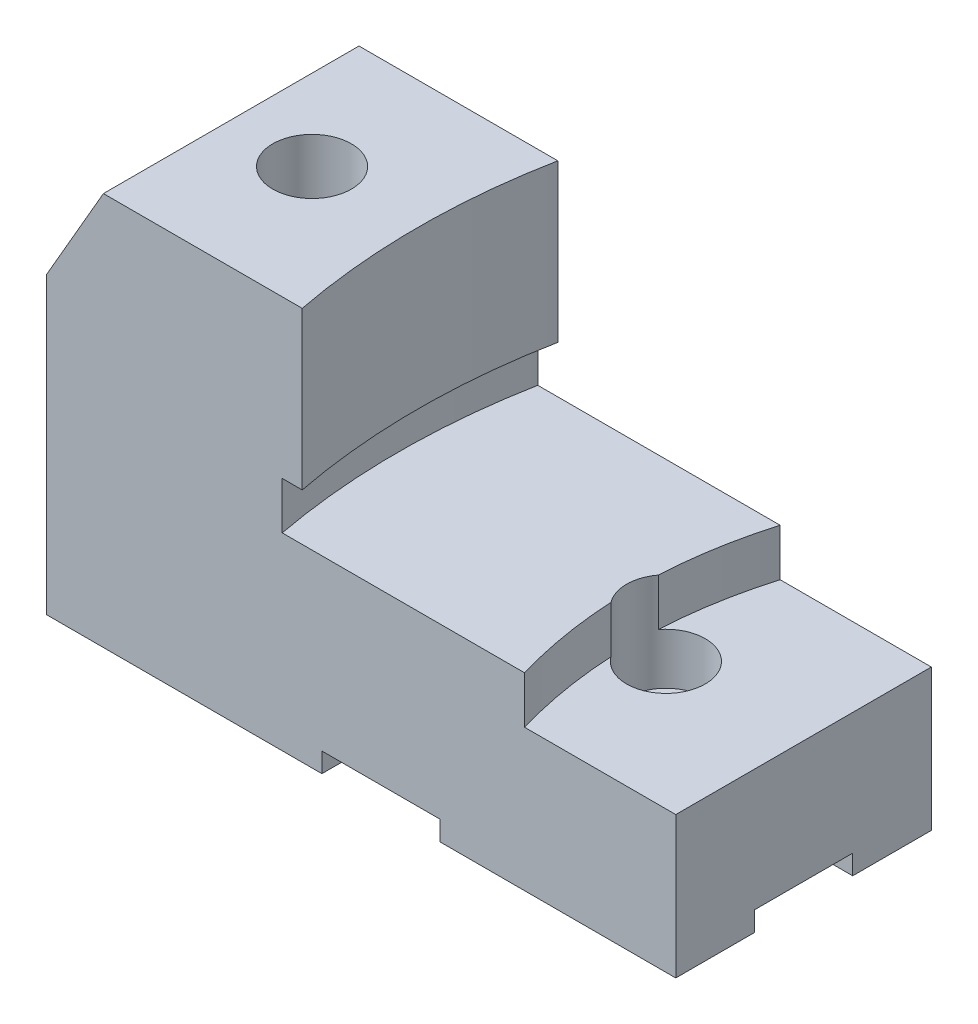
ISO-10303-21;
HEADER;
FILE_DESCRIPTION(('STEP AP214'),'2;1');
FILE_NAME('part.step','',(''),(''),'','','');
FILE_SCHEMA(('AUTOMOTIVE_DESIGN { 1 0 10303 214 1 1 1 1 }'));
ENDSEC;
DATA;
#1=APPLICATION_CONTEXT('core data for automotive mechanical design processes');
#2=APPLICATION_PROTOCOL_DEFINITION('international standard','automotive_design',2000,#1);
#3=PRODUCT_CONTEXT('',#1,'mechanical');
#4=PRODUCT('Part','Part','',(#3));
#5=PRODUCT_RELATED_PRODUCT_CATEGORY('part','',(#4));
#6=PRODUCT_DEFINITION_FORMATION('','',#4);
#7=PRODUCT_DEFINITION_CONTEXT('part definition',#1,'design');
#8=PRODUCT_DEFINITION('design','',#6,#7);
#9=PRODUCT_DEFINITION_SHAPE('','',#8);
#10=(LENGTH_UNIT() NAMED_UNIT(*) SI_UNIT(.MILLI.,.METRE.));
#11=(NAMED_UNIT(*) PLANE_ANGLE_UNIT() SI_UNIT($,.RADIAN.));
#12=(NAMED_UNIT(*) SI_UNIT($,.STERADIAN.) SOLID_ANGLE_UNIT());
#13=UNCERTAINTY_MEASURE_WITH_UNIT(LENGTH_MEASURE(1.E-05),#10,'distance_accuracy_value','');
#14=(GEOMETRIC_REPRESENTATION_CONTEXT(3) GLOBAL_UNCERTAINTY_ASSIGNED_CONTEXT((#13)) GLOBAL_UNIT_ASSIGNED_CONTEXT((#10,
#11,#12)) REPRESENTATION_CONTEXT('',''));
#15=CARTESIAN_POINT('',(0.,0.,0.));
#16=DIRECTION('',(0.,0.,1.));
#17=DIRECTION('',(1.,0.,0.));
#18=AXIS2_PLACEMENT_3D('',#15,#16,#17);
#19=CARTESIAN_POINT('',(-125.,100.,32.5));
#20=DIRECTION('',(0.,-1.,0.));
#21=DIRECTION('',(1.,0.,0.));
#22=AXIS2_PLACEMENT_3D('',#19,#20,#21);
#23=PLANE('',#22);
#24=DIRECTION('',(-1.,0.,0.));
#25=VECTOR('',#24,1.);
#26=CARTESIAN_POINT('',(-125.,100.,-32.5));
#27=LINE('',#26,#25);
#28=CARTESIAN_POINT('',(-60.,100.000006,-32.5));
#29=VERTEX_POINT('',#28);
#30=CARTESIAN_POINT('',(-110.56624327026,100.,-32.5));
#31=VERTEX_POINT('',#30);
#32=EDGE_CURVE('E452',#29,#31,#27,.T.);
#33=ORIENTED_EDGE('',*,*,#32,.T.);
#34=DIRECTION('',(0.,0.,1.));
#35=VECTOR('',#34,1.);
#36=CARTESIAN_POINT('',(-110.566242501029,100.000001332347,-32.55003));
#37=LINE('',#36,#35);
#38=CARTESIAN_POINT('',(-110.566242501029,100.000001332347,32.5));
#39=VERTEX_POINT('',#38);
#40=EDGE_CURVE('E405',#31,#39,#37,.T.);
#41=ORIENTED_EDGE('',*,*,#40,.T.);
#42=DIRECTION('',(-1.,0.,0.));
#43=VECTOR('',#42,1.);
#44=CARTESIAN_POINT('',(-125.,100.,32.5));
#45=LINE('',#44,#43);
#46=CARTESIAN_POINT('',(-60.,100.000006,32.5));
#47=VERTEX_POINT('',#46);
#48=EDGE_CURVE('E418',#47,#39,#45,.T.);
#49=ORIENTED_EDGE('',*,*,#48,.F.);
#50=CARTESIAN_POINT('',(106.864465959652,100.000012,0.));
#51=DIRECTION('',(0.,1.,0.));
#52=DIRECTION('',(-0.981555682115602,0.,-0.191176470588236));
#53=AXIS2_PLACEMENT_3D('',#50,#51,#52);
#54=CIRCLE('',#53,170.);
#55=EDGE_CURVE('E254',#29,#47,#54,.T.);
#56=ORIENTED_EDGE('',*,*,#55,.F.);
#57=EDGE_LOOP('',(#33,#41,#49,#56));
#58=FACE_BOUND('',#57,.T.);
#59=CARTESIAN_POINT('',(-90.,100.,0.));
#60=DIRECTION('',(0.,1.,0.));
#61=DIRECTION('',(0.,0.,1.));
#62=AXIS2_PLACEMENT_3D('',#59,#60,#61);
#63=CIRCLE('',#62,10.);
#64=CARTESIAN_POINT('',(-90.,100.,10.));
#65=VERTEX_POINT('',#64);
#66=EDGE_CURVE('E798',#65,#65,#63,.T.);
#67=ORIENTED_EDGE('',*,*,#66,.F.);
#68=EDGE_LOOP('',(#67));
#69=FACE_BOUND('',#68,.T.);
#70=ADVANCED_FACE('F51',(#58,#69),#23,.F.);
#71=CARTESIAN_POINT('',(-65.09,48.,32.5));
#72=DIRECTION('',(0.,-1.,0.));
#73=DIRECTION('',(0.,0.,-1.));
#74=AXIS2_PLACEMENT_3D('',#71,#72,#73);
#75=PLANE('',#74);
#76=CARTESIAN_POINT('',(0.,48.,0.));
#77=DIRECTION('',(0.,1.,0.));
#78=DIRECTION('',(0.,0.,1.));
#79=AXIS2_PLACEMENT_3D('',#76,#77,#78);
#80=CIRCLE('',#79,10.);
#81=CARTESIAN_POINT('',(-7.97991699709289,48.,-6.02668438857621));
#82=VERTEX_POINT('',#81);
#83=CARTESIAN_POINT('',(-7.97991699709294,48.,6.02668438857625));
#84=VERTEX_POINT('',#83);
#85=EDGE_CURVE('E66',#82,#84,#80,.T.);
#86=ORIENTED_EDGE('',*,*,#85,.F.);
#87=CARTESIAN_POINT('',(106.862057364551,48.,0.));
#88=DIRECTION('',(0.,-1.,0.));
#89=DIRECTION('',(0.,0.,-1.));
#90=AXIS2_PLACEMENT_3D('',#87,#88,#89);
#91=CIRCLE('',#90,115.);
#92=CARTESIAN_POINT('',(-3.45,48.,-32.5));
#93=VERTEX_POINT('',#92);
#94=EDGE_CURVE('E228',#93,#82,#91,.F.);
#95=ORIENTED_EDGE('',*,*,#94,.F.);
#96=DIRECTION('',(-1.,0.,0.));
#97=VECTOR('',#96,1.);
#98=CARTESIAN_POINT('',(-65.09,48.,-32.5));
#99=LINE('',#98,#97);
#100=CARTESIAN_POINT('',(-65.09,48.,-32.5));
#101=VERTEX_POINT('',#100);
#102=EDGE_CURVE('E439',#93,#101,#99,.T.);
#103=ORIENTED_EDGE('',*,*,#102,.T.);
#104=CARTESIAN_POINT('',(106.864465959652,48.,0.));
#105=DIRECTION('',(0.,1.,0.));
#106=DIRECTION('',(0.,0.,1.));
#107=AXIS2_PLACEMENT_3D('',#104,#105,#106);
#108=CIRCLE('',#107,174.998823891674);
#109=CARTESIAN_POINT('',(-65.09,48.,32.5));
#110=VERTEX_POINT('',#109);
#111=EDGE_CURVE('E236',#101,#110,#108,.T.);
#112=ORIENTED_EDGE('',*,*,#111,.T.);
#113=DIRECTION('',(-1.,0.,0.));
#114=VECTOR('',#113,1.);
#115=CARTESIAN_POINT('',(-65.09,48.,32.5));
#116=LINE('',#115,#114);
#117=CARTESIAN_POINT('',(-3.45,48.,32.5));
#118=VERTEX_POINT('',#117);
#119=EDGE_CURVE('E594',#118,#110,#116,.T.);
#120=ORIENTED_EDGE('',*,*,#119,.F.);
#121=EDGE_CURVE('E230',#84,#118,#91,.F.);
#122=ORIENTED_EDGE('',*,*,#121,.F.);
#123=EDGE_LOOP('',(#86,#95,#103,#112,#120,#122));
#124=FACE_BOUND('',#123,.T.);
#125=ADVANCED_FACE('F223',(#124),#75,.F.);
#126=CARTESIAN_POINT('',(106.862057364551,113.16883308878,0.));
#127=DIRECTION('',(0.,-1.,0.));
#128=DIRECTION('',(0.,0.,-1.));
#129=AXIS2_PLACEMENT_3D('',#126,#127,#128);
#130=CYLINDRICAL_SURFACE('',#129,115.);
#131=ORIENTED_EDGE('',*,*,#94,.T.);
#132=DIRECTION('',(0.,1.,0.));
#133=VECTOR('',#132,1.);
#134=CARTESIAN_POINT('',(-7.97991699709289,35.5,-6.02668438857621));
#135=LINE('',#134,#133);
#136=CARTESIAN_POINT('',(-7.97991699709294,36.,-6.02668438857625));
#137=VERTEX_POINT('',#136);
#138=EDGE_CURVE('E12',#82,#137,#135,.F.);
#139=ORIENTED_EDGE('',*,*,#138,.T.);
#140=CARTESIAN_POINT('',(106.862057364551,36.,0.));
#141=DIRECTION('',(0.,-1.,0.));
#142=DIRECTION('',(0.,0.,-1.));
#143=AXIS2_PLACEMENT_3D('',#140,#141,#142);
#144=CIRCLE('',#143,115.);
#145=CARTESIAN_POINT('',(-3.45,36.,-32.5));
#146=VERTEX_POINT('',#145);
#147=EDGE_CURVE('E250',#137,#146,#144,.T.);
#148=ORIENTED_EDGE('',*,*,#147,.T.);
#149=DIRECTION('',(0.,1.,0.));
#150=VECTOR('',#149,1.);
#151=CARTESIAN_POINT('',(-3.45,48.,-32.5));
#152=LINE('',#151,#150);
#153=EDGE_CURVE('E232',#146,#93,#152,.T.);
#154=ORIENTED_EDGE('',*,*,#153,.T.);
#155=EDGE_LOOP('',(#131,#139,#148,#154));
#156=FACE_BOUND('',#155,.T.);
#157=ADVANCED_FACE('F231',(#156),#130,.F.);
#158=CARTESIAN_POINT('',(35.,0.,32.5));
#159=DIRECTION('',(0.,1.,0.));
#160=DIRECTION('',(-1.,0.,0.));
#161=AXIS2_PLACEMENT_3D('',#158,#159,#160);
#162=PLANE('',#161);
#163=DIRECTION('',(1.,0.,0.));
#164=VECTOR('',#163,1.);
#165=CARTESIAN_POINT('',(-125.,0.,-12.5));
#166=LINE('',#165,#164);
#167=CARTESIAN_POINT('',(-25.,0.,-12.5));
#168=VERTEX_POINT('',#167);
#169=CARTESIAN_POINT('',(35.,0.,-12.5));
#170=VERTEX_POINT('',#169);
#171=EDGE_CURVE('E368',#168,#170,#166,.T.);
#172=ORIENTED_EDGE('',*,*,#171,.F.);
#173=DIRECTION('',(0.,0.,1.));
#174=VECTOR('',#173,1.);
#175=CARTESIAN_POINT('',(-25.,0.,-32.55003));
#176=LINE('',#175,#174);
#177=CARTESIAN_POINT('',(-25.,0.,-32.5));
#178=VERTEX_POINT('',#177);
#179=EDGE_CURVE('E395',#178,#168,#176,.T.);
#180=ORIENTED_EDGE('',*,*,#179,.F.);
#181=DIRECTION('',(1.,0.,0.));
#182=VECTOR('',#181,1.);
#183=CARTESIAN_POINT('',(35.,0.,-32.5));
#184=LINE('',#183,#182);
#185=CARTESIAN_POINT('',(35.,0.,-32.5));
#186=VERTEX_POINT('',#185);
#187=EDGE_CURVE('E448',#178,#186,#184,.T.);
#188=ORIENTED_EDGE('',*,*,#187,.T.);
#189=DIRECTION('',(0.,0.,-1.));
#190=VECTOR('',#189,1.);
#191=CARTESIAN_POINT('',(35.,0.,32.5));
#192=LINE('',#191,#190);
#193=EDGE_CURVE('E433',#170,#186,#192,.T.);
#194=ORIENTED_EDGE('',*,*,#193,.F.);
#195=EDGE_LOOP('',(#172,#180,#188,#194));
#196=FACE_BOUND('',#195,.T.);
#197=ADVANCED_FACE('F293',(#196),#162,.F.);
#198=CARTESIAN_POINT('',(-125.,0.,-12.5));
#199=VERTEX_POINT('',#198);
#200=CARTESIAN_POINT('',(-55.,0.,-12.5));
#201=VERTEX_POINT('',#200);
#202=EDGE_CURVE('E73',#199,#201,#166,.T.);
#203=ORIENTED_EDGE('',*,*,#202,.F.);
#204=DIRECTION('',(0.,0.,-1.));
#205=VECTOR('',#204,1.);
#206=CARTESIAN_POINT('',(-125.,0.,32.5));
#207=LINE('',#206,#205);
#208=CARTESIAN_POINT('',(-125.,0.,-32.5));
#209=VERTEX_POINT('',#208);
#210=EDGE_CURVE('E459',#199,#209,#207,.T.);
#211=ORIENTED_EDGE('',*,*,#210,.T.);
#212=CARTESIAN_POINT('',(-55.,0.,-32.5));
#213=VERTEX_POINT('',#212);
#214=EDGE_CURVE('E455',#209,#213,#184,.T.);
#215=ORIENTED_EDGE('',*,*,#214,.T.);
#216=DIRECTION('',(0.,0.,1.));
#217=VECTOR('',#216,1.);
#218=CARTESIAN_POINT('',(-55.,0.,-32.55003));
#219=LINE('',#218,#217);
#220=EDGE_CURVE('E398',#213,#201,#219,.T.);
#221=ORIENTED_EDGE('',*,*,#220,.T.);
#222=EDGE_LOOP('',(#203,#211,#215,#221));
#223=FACE_BOUND('',#222,.T.);
#224=ADVANCED_FACE('F478',(#223),#162,.F.);
#225=CARTESIAN_POINT('',(35.,36.,32.5));
#226=DIRECTION('',(-1.,0.,0.));
#227=DIRECTION('',(0.,-1.,0.));
#228=AXIS2_PLACEMENT_3D('',#225,#226,#227);
#229=PLANE('',#228);
#230=DIRECTION('',(0.,-1.,0.));
#231=VECTOR('',#230,1.);
#232=CARTESIAN_POINT('',(35.,0.,12.5));
#233=LINE('',#232,#231);
#234=CARTESIAN_POINT('',(35.,5.,12.5));
#235=VERTEX_POINT('',#234);
#236=CARTESIAN_POINT('',(35.,0.,12.5));
#237=VERTEX_POINT('',#236);
#238=EDGE_CURVE('E333',#235,#237,#233,.T.);
#239=ORIENTED_EDGE('',*,*,#238,.F.);
#240=DIRECTION('',(0.,0.,1.));
#241=VECTOR('',#240,1.);
#242=CARTESIAN_POINT('',(35.,5.,12.5));
#243=LINE('',#242,#241);
#244=CARTESIAN_POINT('',(35.,5.,-12.5));
#245=VERTEX_POINT('',#244);
#246=EDGE_CURVE('E349',#245,#235,#243,.T.);
#247=ORIENTED_EDGE('',*,*,#246,.F.);
#248=DIRECTION('',(0.,1.,0.));
#249=VECTOR('',#248,1.);
#250=CARTESIAN_POINT('',(35.,0.,-12.5));
#251=LINE('',#250,#249);
#252=EDGE_CURVE('E340',#170,#245,#251,.T.);
#253=ORIENTED_EDGE('',*,*,#252,.F.);
#254=ORIENTED_EDGE('',*,*,#193,.T.);
#255=DIRECTION('',(0.,1.,0.));
#256=VECTOR('',#255,1.);
#257=CARTESIAN_POINT('',(35.,36.,-32.5));
#258=LINE('',#257,#256);
#259=CARTESIAN_POINT('',(35.,36.,-32.5));
#260=VERTEX_POINT('',#259);
#261=EDGE_CURVE('E432',#186,#260,#258,.T.);
#262=ORIENTED_EDGE('',*,*,#261,.T.);
#263=DIRECTION('',(0.,0.,-1.));
#264=VECTOR('',#263,1.);
#265=CARTESIAN_POINT('',(35.,36.,32.5));
#266=LINE('',#265,#264);
#267=CARTESIAN_POINT('',(35.,36.,32.5));
#268=VERTEX_POINT('',#267);
#269=EDGE_CURVE('E314',#268,#260,#266,.T.);
#270=ORIENTED_EDGE('',*,*,#269,.F.);
#271=DIRECTION('',(0.,1.,0.));
#272=VECTOR('',#271,1.);
#273=CARTESIAN_POINT('',(35.,36.,32.5));
#274=LINE('',#273,#272);
#275=CARTESIAN_POINT('',(35.,0.,32.5));
#276=VERTEX_POINT('',#275);
#277=EDGE_CURVE('E262',#276,#268,#274,.T.);
#278=ORIENTED_EDGE('',*,*,#277,.F.);
#279=EDGE_CURVE('E453',#276,#237,#192,.T.);
#280=ORIENTED_EDGE('',*,*,#279,.T.);
#281=EDGE_LOOP('',(#239,#247,#253,#254,#262,#270,#278,#280));
#282=FACE_BOUND('',#281,.T.);
#283=ADVANCED_FACE('F52',(#282),#229,.F.);
#284=CARTESIAN_POINT('',(-55.,0.,-32.55003));
#285=DIRECTION('',(-1.,0.,0.));
#286=DIRECTION('',(0.,0.,1.));
#287=AXIS2_PLACEMENT_3D('',#284,#285,#286);
#288=PLANE('',#287);
#289=CARTESIAN_POINT('',(-55.,0.,12.5));
#290=VERTEX_POINT('',#289);
#291=CARTESIAN_POINT('',(-55.,0.,32.5));
#292=VERTEX_POINT('',#291);
#293=EDGE_CURVE('E383',#290,#292,#219,.T.);
#294=ORIENTED_EDGE('',*,*,#293,.F.);
#295=DIRECTION('',(0.,1.,0.));
#296=VECTOR('',#295,1.);
#297=CARTESIAN_POINT('',(-55.,0.,12.5));
#298=LINE('',#297,#296);
#299=CARTESIAN_POINT('',(-55.,4.99999999999996,12.5));
#300=VERTEX_POINT('',#299);
#301=EDGE_CURVE('E373',#290,#300,#298,.T.);
#302=ORIENTED_EDGE('',*,*,#301,.T.);
#303=DIRECTION('',(0.,0.,1.));
#304=VECTOR('',#303,1.);
#305=CARTESIAN_POINT('',(-55.,4.99999999999998,-32.55003));
#306=LINE('',#305,#304);
#307=CARTESIAN_POINT('',(-55.,4.99999999999998,32.5));
#308=VERTEX_POINT('',#307);
#309=EDGE_CURVE('E388',#300,#308,#306,.T.);
#310=ORIENTED_EDGE('',*,*,#309,.T.);
#311=DIRECTION('',(0.,-1.,0.));
#312=VECTOR('',#311,1.);
#313=CARTESIAN_POINT('',(-55.,0.,32.5));
#314=LINE('',#313,#312);
#315=EDGE_CURVE('E376',#308,#292,#314,.T.);
#316=ORIENTED_EDGE('',*,*,#315,.T.);
#317=EDGE_LOOP('',(#294,#302,#310,#316));
#318=FACE_BOUND('',#317,.T.);
#319=ADVANCED_FACE('F550',(#318),#288,.F.);
#320=CARTESIAN_POINT('',(-25.,0.,-32.55003));
#321=DIRECTION('',(1.,0.,0.));
#322=DIRECTION('',(0.,0.,-1.));
#323=AXIS2_PLACEMENT_3D('',#320,#321,#322);
#324=PLANE('',#323);
#325=DIRECTION('',(0.,0.,1.));
#326=VECTOR('',#325,1.);
#327=CARTESIAN_POINT('',(-25.,4.99999999999998,-32.55003));
#328=LINE('',#327,#326);
#329=CARTESIAN_POINT('',(-25.,4.99999999999997,12.5));
#330=VERTEX_POINT('',#329);
#331=CARTESIAN_POINT('',(-25.,4.99999999999998,32.5));
#332=VERTEX_POINT('',#331);
#333=EDGE_CURVE('E393',#330,#332,#328,.T.);
#334=ORIENTED_EDGE('',*,*,#333,.F.);
#335=DIRECTION('',(0.,-1.,0.));
#336=VECTOR('',#335,1.);
#337=CARTESIAN_POINT('',(-25.,0.,12.5));
#338=LINE('',#337,#336);
#339=CARTESIAN_POINT('',(-25.,0.,12.5));
#340=VERTEX_POINT('',#339);
#341=EDGE_CURVE('E323',#330,#340,#338,.T.);
#342=ORIENTED_EDGE('',*,*,#341,.T.);
#343=CARTESIAN_POINT('',(-25.,0.,32.5));
#344=VERTEX_POINT('',#343);
#345=EDGE_CURVE('E399',#340,#344,#176,.T.);
#346=ORIENTED_EDGE('',*,*,#345,.T.);
#347=DIRECTION('',(0.,1.,0.));
#348=VECTOR('',#347,1.);
#349=CARTESIAN_POINT('',(-25.,0.,32.5));
#350=LINE('',#349,#348);
#351=EDGE_CURVE('E378',#344,#332,#350,.T.);
#352=ORIENTED_EDGE('',*,*,#351,.T.);
#353=EDGE_LOOP('',(#334,#342,#346,#352));
#354=FACE_BOUND('',#353,.T.);
#355=ADVANCED_FACE('F541',(#354),#324,.F.);
#356=ORIENTED_EDGE('',*,*,#345,.F.);
#357=DIRECTION('',(1.,0.,0.));
#358=VECTOR('',#357,1.);
#359=CARTESIAN_POINT('',(-125.,0.,12.5));
#360=LINE('',#359,#358);
#361=EDGE_CURVE('E354',#340,#237,#360,.T.);
#362=ORIENTED_EDGE('',*,*,#361,.T.);
#363=ORIENTED_EDGE('',*,*,#279,.F.);
#364=DIRECTION('',(1.,0.,0.));
#365=VECTOR('',#364,1.);
#366=CARTESIAN_POINT('',(35.,0.,32.5));
#367=LINE('',#366,#365);
#368=EDGE_CURVE('E421',#344,#276,#367,.T.);
#369=ORIENTED_EDGE('',*,*,#368,.F.);
#370=EDGE_LOOP('',(#356,#362,#363,#369));
#371=FACE_BOUND('',#370,.T.);
#372=ADVANCED_FACE('F281',(#371),#162,.F.);
#373=CARTESIAN_POINT('',(0.,0.,32.5));
#374=DIRECTION('',(0.,0.,-1.));
#375=DIRECTION('',(-1.,0.,0.));
#376=AXIS2_PLACEMENT_3D('',#373,#374,#375);
#377=PLANE('',#376);
#378=ORIENTED_EDGE('',*,*,#315,.F.);
#379=DIRECTION('',(-1.,0.,0.));
#380=VECTOR('',#379,1.);
#381=CARTESIAN_POINT('',(-55.,4.99999999999998,32.5));
#382=LINE('',#381,#380);
#383=EDGE_CURVE('E385',#332,#308,#382,.T.);
#384=ORIENTED_EDGE('',*,*,#383,.F.);
#385=ORIENTED_EDGE('',*,*,#351,.F.);
#386=ORIENTED_EDGE('',*,*,#368,.T.);
#387=ORIENTED_EDGE('',*,*,#277,.T.);
#388=DIRECTION('',(-1.,0.,0.));
#389=VECTOR('',#388,1.);
#390=CARTESIAN_POINT('',(-3.45,36.,32.5));
#391=LINE('',#390,#389);
#392=CARTESIAN_POINT('',(-3.45,36.,32.5));
#393=VERTEX_POINT('',#392);
#394=EDGE_CURVE('E527',#268,#393,#391,.T.);
#395=ORIENTED_EDGE('',*,*,#394,.T.);
#396=DIRECTION('',(0.,1.,0.));
#397=VECTOR('',#396,1.);
#398=CARTESIAN_POINT('',(-3.45,48.,32.5));
#399=LINE('',#398,#397);
#400=EDGE_CURVE('E529',#393,#118,#399,.T.);
#401=ORIENTED_EDGE('',*,*,#400,.T.);
#402=ORIENTED_EDGE('',*,*,#119,.T.);
#403=DIRECTION('',(0.,1.,0.));
#404=VECTOR('',#403,1.);
#405=CARTESIAN_POINT('',(-65.09,60.,32.5));
#406=LINE('',#405,#404);
#407=CARTESIAN_POINT('',(-65.09,60.,32.5));
#408=VERTEX_POINT('',#407);
#409=EDGE_CURVE('E591',#110,#408,#406,.T.);
#410=ORIENTED_EDGE('',*,*,#409,.T.);
#411=DIRECTION('',(1.,0.,0.));
#412=VECTOR('',#411,1.);
#413=CARTESIAN_POINT('',(-60.,60.,32.5));
#414=LINE('',#413,#412);
#415=CARTESIAN_POINT('',(-60.,60.,32.5));
#416=VERTEX_POINT('',#415);
#417=EDGE_CURVE('E427',#408,#416,#414,.T.);
#418=ORIENTED_EDGE('',*,*,#417,.T.);
#419=DIRECTION('',(0.,1.,0.));
#420=VECTOR('',#419,1.);
#421=CARTESIAN_POINT('',(-60.,100.,32.5));
#422=LINE('',#421,#420);
#423=EDGE_CURVE('E430',#416,#47,#422,.T.);
#424=ORIENTED_EDGE('',*,*,#423,.T.);
#425=ORIENTED_EDGE('',*,*,#48,.T.);
#426=DIRECTION('',(0.499999999999995,0.866025403784442,0.));
#427=VECTOR('',#426,1.);
#428=CARTESIAN_POINT('',(-110.566242501029,100.000001332347,32.5));
#429=LINE('',#428,#427);
#430=CARTESIAN_POINT('',(-125.,75.,32.5));
#431=VERTEX_POINT('',#430);
#432=EDGE_CURVE('E386',#431,#39,#429,.T.);
#433=ORIENTED_EDGE('',*,*,#432,.F.);
#434=DIRECTION('',(0.,-1.,0.));
#435=VECTOR('',#434,1.);
#436=CARTESIAN_POINT('',(-125.,0.,32.5));
#437=LINE('',#436,#435);
#438=CARTESIAN_POINT('',(-125.,0.,32.5));
#439=VERTEX_POINT('',#438);
#440=EDGE_CURVE('E417',#431,#439,#437,.T.);
#441=ORIENTED_EDGE('',*,*,#440,.T.);
#442=EDGE_CURVE('E424',#439,#292,#367,.T.);
#443=ORIENTED_EDGE('',*,*,#442,.T.);
#444=EDGE_LOOP('',(#378,#384,#385,#386,#387,#395,#401,#402,#410,#418,#424,#425,#433,#441,#443));
#445=FACE_BOUND('',#444,.T.);
#446=ADVANCED_FACE('F280',(#445),#377,.F.);
#447=CARTESIAN_POINT('',(-125.,0.,32.5));
#448=DIRECTION('',(1.,0.,0.));
#449=DIRECTION('',(0.,0.,-1.));
#450=AXIS2_PLACEMENT_3D('',#447,#448,#449);
#451=PLANE('',#450);
#452=DIRECTION('',(0.,0.,1.));
#453=VECTOR('',#452,1.);
#454=CARTESIAN_POINT('',(-125.,4.99999999999994,12.5));
#455=LINE('',#454,#453);
#456=CARTESIAN_POINT('',(-125.,4.99999999999994,-12.5));
#457=VERTEX_POINT('',#456);
#458=CARTESIAN_POINT('',(-125.,4.99999999999994,12.5));
#459=VERTEX_POINT('',#458);
#460=EDGE_CURVE('E351',#457,#459,#455,.T.);
#461=ORIENTED_EDGE('',*,*,#460,.T.);
#462=DIRECTION('',(0.,-1.,0.));
#463=VECTOR('',#462,1.);
#464=CARTESIAN_POINT('',(-125.,0.,12.5));
#465=LINE('',#464,#463);
#466=CARTESIAN_POINT('',(-125.,0.,12.5));
#467=VERTEX_POINT('',#466);
#468=EDGE_CURVE('E341',#459,#467,#465,.T.);
#469=ORIENTED_EDGE('',*,*,#468,.T.);
#470=EDGE_CURVE('E423',#439,#467,#207,.T.);
#471=ORIENTED_EDGE('',*,*,#470,.F.);
#472=ORIENTED_EDGE('',*,*,#440,.F.);
#473=DIRECTION('',(0.,0.,1.));
#474=VECTOR('',#473,1.);
#475=CARTESIAN_POINT('',(-125.,75.,-32.55003));
#476=LINE('',#475,#474);
#477=CARTESIAN_POINT('',(-125.,75.,-32.5));
#478=VERTEX_POINT('',#477);
#479=EDGE_CURVE('E242',#478,#431,#476,.T.);
#480=ORIENTED_EDGE('',*,*,#479,.F.);
#481=DIRECTION('',(0.,-1.,0.));
#482=VECTOR('',#481,1.);
#483=CARTESIAN_POINT('',(-125.,0.,-32.5));
#484=LINE('',#483,#482);
#485=EDGE_CURVE('E449',#478,#209,#484,.T.);
#486=ORIENTED_EDGE('',*,*,#485,.T.);
#487=ORIENTED_EDGE('',*,*,#210,.F.);
#488=DIRECTION('',(0.,1.,0.));
#489=VECTOR('',#488,1.);
#490=CARTESIAN_POINT('',(-125.,0.,-12.5));
#491=LINE('',#490,#489);
#492=EDGE_CURVE('E347',#199,#457,#491,.T.);
#493=ORIENTED_EDGE('',*,*,#492,.T.);
#494=EDGE_LOOP('',(#461,#469,#471,#472,#480,#486,#487,#493));
#495=FACE_BOUND('',#494,.T.);
#496=ADVANCED_FACE('F278',(#495),#451,.F.);
#497=CARTESIAN_POINT('',(-3.45,36.,32.5));
#498=DIRECTION('',(0.,-1.,0.));
#499=DIRECTION('',(0.,0.,-1.));
#500=AXIS2_PLACEMENT_3D('',#497,#498,#499);
#501=PLANE('',#500);
#502=ORIENTED_EDGE('',*,*,#147,.F.);
#503=CARTESIAN_POINT('',(0.,36.,0.));
#504=DIRECTION('',(0.,-1.,0.));
#505=DIRECTION('',(0.,0.,-1.));
#506=AXIS2_PLACEMENT_3D('',#503,#504,#505);
#507=CIRCLE('',#506,10.);
#508=CARTESIAN_POINT('',(-7.97991699709294,36.,6.02668438857625));
#509=VERTEX_POINT('',#508);
#510=EDGE_CURVE('E217',#137,#509,#507,.T.);
#511=ORIENTED_EDGE('',*,*,#510,.T.);
#512=EDGE_CURVE('E241',#393,#509,#144,.T.);
#513=ORIENTED_EDGE('',*,*,#512,.F.);
#514=ORIENTED_EDGE('',*,*,#394,.F.);
#515=ORIENTED_EDGE('',*,*,#269,.T.);
#516=DIRECTION('',(-1.,0.,0.));
#517=VECTOR('',#516,1.);
#518=CARTESIAN_POINT('',(-3.45,36.,-32.5));
#519=LINE('',#518,#517);
#520=EDGE_CURVE('E440',#260,#146,#519,.T.);
#521=ORIENTED_EDGE('',*,*,#520,.T.);
#522=EDGE_LOOP('',(#502,#511,#513,#514,#515,#521));
#523=FACE_BOUND('',#522,.T.);
#524=ADVANCED_FACE('F295',(#523),#501,.F.);
#525=CARTESIAN_POINT('',(-60.,60.,32.5));
#526=DIRECTION('',(0.,1.,0.));
#527=DIRECTION('',(0.,0.,1.));
#528=AXIS2_PLACEMENT_3D('',#525,#526,#527);
#529=PLANE('',#528);
#530=DIRECTION('',(1.,0.,0.));
#531=VECTOR('',#530,1.);
#532=CARTESIAN_POINT('',(-60.,60.,-32.5));
#533=LINE('',#532,#531);
#534=CARTESIAN_POINT('',(-65.09,60.,-32.5));
#535=VERTEX_POINT('',#534);
#536=CARTESIAN_POINT('',(-60.,60.,-32.5));
#537=VERTEX_POINT('',#536);
#538=EDGE_CURVE('E443',#535,#537,#533,.T.);
#539=ORIENTED_EDGE('',*,*,#538,.T.);
#540=CARTESIAN_POINT('',(106.864465959652,60.,0.));
#541=DIRECTION('',(0.,1.,0.));
#542=DIRECTION('',(-1.,0.,0.));
#543=AXIS2_PLACEMENT_3D('',#540,#541,#542);
#544=CIRCLE('',#543,170.);
#545=EDGE_CURVE('E249',#537,#416,#544,.T.);
#546=ORIENTED_EDGE('',*,*,#545,.T.);
#547=ORIENTED_EDGE('',*,*,#417,.F.);
#548=CARTESIAN_POINT('',(106.864465959652,60.,0.));
#549=DIRECTION('',(0.,1.,0.));
#550=DIRECTION('',(0.,0.,1.));
#551=AXIS2_PLACEMENT_3D('',#548,#549,#550);
#552=CIRCLE('',#551,174.998823891674);
#553=EDGE_CURVE('E237',#535,#408,#552,.T.);
#554=ORIENTED_EDGE('',*,*,#553,.F.);
#555=EDGE_LOOP('',(#539,#546,#547,#554));
#556=FACE_BOUND('',#555,.T.);
#557=ADVANCED_FACE('F288',(#556),#529,.F.);
#558=ORIENTED_EDGE('',*,*,#470,.T.);
#559=EDGE_CURVE('E367',#467,#290,#360,.T.);
#560=ORIENTED_EDGE('',*,*,#559,.T.);
#561=ORIENTED_EDGE('',*,*,#293,.T.);
#562=ORIENTED_EDGE('',*,*,#442,.F.);
#563=EDGE_LOOP('',(#558,#560,#561,#562));
#564=FACE_BOUND('',#563,.T.);
#565=ADVANCED_FACE('F285',(#564),#162,.F.);
#566=CARTESIAN_POINT('',(0.,0.,-32.5));
#567=DIRECTION('',(0.,0.,-1.));
#568=DIRECTION('',(-1.,0.,0.));
#569=AXIS2_PLACEMENT_3D('',#566,#567,#568);
#570=PLANE('',#569);
#571=DIRECTION('',(0.,1.,0.));
#572=VECTOR('',#571,1.);
#573=CARTESIAN_POINT('',(-55.,0.,-32.5));
#574=LINE('',#573,#572);
#575=CARTESIAN_POINT('',(-55.,4.99999999999998,-32.5));
#576=VERTEX_POINT('',#575);
#577=EDGE_CURVE('E318',#213,#576,#574,.T.);
#578=ORIENTED_EDGE('',*,*,#577,.F.);
#579=ORIENTED_EDGE('',*,*,#214,.F.);
#580=ORIENTED_EDGE('',*,*,#485,.F.);
#581=DIRECTION('',(-0.499999999999995,-0.866025403784442,0.));
#582=VECTOR('',#581,1.);
#583=CARTESIAN_POINT('',(-126.225952641917,72.8765877365266,-32.5));
#584=LINE('',#583,#582);
#585=EDGE_CURVE('E310',#31,#478,#584,.T.);
#586=ORIENTED_EDGE('',*,*,#585,.F.);
#587=ORIENTED_EDGE('',*,*,#32,.F.);
#588=DIRECTION('',(0.,1.,0.));
#589=VECTOR('',#588,1.);
#590=CARTESIAN_POINT('',(-60.,100.,-32.5));
#591=LINE('',#590,#589);
#592=EDGE_CURVE('E450',#537,#29,#591,.T.);
#593=ORIENTED_EDGE('',*,*,#592,.F.);
#594=ORIENTED_EDGE('',*,*,#538,.F.);
#595=DIRECTION('',(0.,1.,0.));
#596=VECTOR('',#595,1.);
#597=CARTESIAN_POINT('',(-65.09,60.,-32.5));
#598=LINE('',#597,#596);
#599=EDGE_CURVE('E445',#101,#535,#598,.T.);
#600=ORIENTED_EDGE('',*,*,#599,.F.);
#601=ORIENTED_EDGE('',*,*,#102,.F.);
#602=ORIENTED_EDGE('',*,*,#153,.F.);
#603=ORIENTED_EDGE('',*,*,#520,.F.);
#604=ORIENTED_EDGE('',*,*,#261,.F.);
#605=ORIENTED_EDGE('',*,*,#187,.F.);
#606=DIRECTION('',(0.,-1.,0.));
#607=VECTOR('',#606,1.);
#608=CARTESIAN_POINT('',(-25.,0.,-32.5));
#609=LINE('',#608,#607);
#610=CARTESIAN_POINT('',(-25.,4.99999999999998,-32.5));
#611=VERTEX_POINT('',#610);
#612=EDGE_CURVE('E313',#611,#178,#609,.T.);
#613=ORIENTED_EDGE('',*,*,#612,.F.);
#614=DIRECTION('',(1.,0.,0.));
#615=VECTOR('',#614,1.);
#616=CARTESIAN_POINT('',(0.,4.99999999999998,-32.5));
#617=LINE('',#616,#615);
#618=EDGE_CURVE('E320',#576,#611,#617,.T.);
#619=ORIENTED_EDGE('',*,*,#618,.F.);
#620=EDGE_LOOP('',(#578,#579,#580,#586,#587,#593,#594,#600,#601,#602,#603,#604,#605,#613,#619));
#621=FACE_BOUND('',#620,.T.);
#622=ADVANCED_FACE('F273',(#621),#570,.T.);
#623=CARTESIAN_POINT('',(106.864465959652,60.,0.));
#624=DIRECTION('',(0.,1.,0.));
#625=DIRECTION('',(-1.,0.,0.));
#626=AXIS2_PLACEMENT_3D('',#623,#624,#625);
#627=CYLINDRICAL_SURFACE('',#626,170.);
#628=ORIENTED_EDGE('',*,*,#55,.T.);
#629=ORIENTED_EDGE('',*,*,#423,.F.);
#630=ORIENTED_EDGE('',*,*,#545,.F.);
#631=ORIENTED_EDGE('',*,*,#592,.T.);
#632=EDGE_LOOP('',(#628,#629,#630,#631));
#633=FACE_BOUND('',#632,.T.);
#634=ADVANCED_FACE('F263',(#633),#627,.F.);
#635=CARTESIAN_POINT('',(106.864465959652,125.071254138969,0.));
#636=DIRECTION('',(0.,-1.,0.));
#637=DIRECTION('',(0.,0.,-1.));
#638=AXIS2_PLACEMENT_3D('',#635,#636,#637);
#639=CYLINDRICAL_SURFACE('',#638,174.998823891674);
#640=ORIENTED_EDGE('',*,*,#553,.T.);
#641=ORIENTED_EDGE('',*,*,#409,.F.);
#642=ORIENTED_EDGE('',*,*,#111,.F.);
#643=ORIENTED_EDGE('',*,*,#599,.T.);
#644=EDGE_LOOP('',(#640,#641,#642,#643));
#645=FACE_BOUND('',#644,.T.);
#646=ADVANCED_FACE('F274',(#645),#639,.F.);
#647=ORIENTED_EDGE('',*,*,#512,.T.);
#648=DIRECTION('',(0.,1.,0.));
#649=VECTOR('',#648,1.);
#650=CARTESIAN_POINT('',(-7.97991699709289,35.5,6.02668438857621));
#651=LINE('',#650,#649);
#652=EDGE_CURVE('E56',#509,#84,#651,.T.);
#653=ORIENTED_EDGE('',*,*,#652,.T.);
#654=ORIENTED_EDGE('',*,*,#121,.T.);
#655=ORIENTED_EDGE('',*,*,#400,.F.);
#656=EDGE_LOOP('',(#647,#653,#654,#655));
#657=FACE_BOUND('',#656,.T.);
#658=ADVANCED_FACE('F329',(#657),#130,.F.);
#659=CARTESIAN_POINT('',(-110.566242501029,100.000001332347,-32.55003));
#660=DIRECTION('',(0.866025403784442,-0.499999999999995,0.));
#661=DIRECTION('',(0.499999999999995,0.866025403784442,0.));
#662=AXIS2_PLACEMENT_3D('',#659,#660,#661);
#663=PLANE('',#662);
#664=ORIENTED_EDGE('',*,*,#585,.T.);
#665=ORIENTED_EDGE('',*,*,#479,.T.);
#666=ORIENTED_EDGE('',*,*,#432,.T.);
#667=ORIENTED_EDGE('',*,*,#40,.F.);
#668=EDGE_LOOP('',(#664,#665,#666,#667));
#669=FACE_BOUND('',#668,.T.);
#670=ADVANCED_FACE('F408',(#669),#663,.F.);
#671=CARTESIAN_POINT('',(-55.,4.99999999999996,-12.5));
#672=VERTEX_POINT('',#671);
#673=EDGE_CURVE('E387',#576,#672,#306,.T.);
#674=ORIENTED_EDGE('',*,*,#673,.T.);
#675=DIRECTION('',(0.,-1.,0.));
#676=VECTOR('',#675,1.);
#677=CARTESIAN_POINT('',(-55.,0.,-12.5));
#678=LINE('',#677,#676);
#679=EDGE_CURVE('E363',#672,#201,#678,.T.);
#680=ORIENTED_EDGE('',*,*,#679,.T.);
#681=ORIENTED_EDGE('',*,*,#220,.F.);
#682=ORIENTED_EDGE('',*,*,#577,.T.);
#683=EDGE_LOOP('',(#674,#680,#681,#682));
#684=FACE_BOUND('',#683,.T.);
#685=ADVANCED_FACE('F481',(#684),#288,.F.);
#686=CARTESIAN_POINT('',(-55.,4.99999999999998,-32.55003));
#687=DIRECTION('',(0.,1.,0.));
#688=DIRECTION('',(0.,0.,1.));
#689=AXIS2_PLACEMENT_3D('',#686,#687,#688);
#690=PLANE('',#689);
#691=CARTESIAN_POINT('',(-90.,4.99999999999998,0.));
#692=DIRECTION('',(0.,1.,0.));
#693=DIRECTION('',(0.,0.,1.));
#694=AXIS2_PLACEMENT_3D('',#691,#692,#693);
#695=CIRCLE('',#694,4.5);
#696=CARTESIAN_POINT('',(-90.,4.99999999999998,4.5));
#697=VERTEX_POINT('',#696);
#698=EDGE_CURVE('E233',#697,#697,#695,.T.);
#699=ORIENTED_EDGE('',*,*,#698,.T.);
#700=EDGE_LOOP('',(#699));
#701=FACE_BOUND('',#700,.T.);
#702=CARTESIAN_POINT('',(0.,4.99999999999998,0.));
#703=DIRECTION('',(0.,1.,0.));
#704=DIRECTION('',(0.,0.,1.));
#705=AXIS2_PLACEMENT_3D('',#702,#703,#704);
#706=CIRCLE('',#705,4.50000000000001);
#707=CARTESIAN_POINT('',(0.,4.99999999999998,4.50000000000001));
#708=VERTEX_POINT('',#707);
#709=EDGE_CURVE('E335',#708,#708,#706,.T.);
#710=ORIENTED_EDGE('',*,*,#709,.T.);
#711=EDGE_LOOP('',(#710));
#712=FACE_BOUND('',#711,.T.);
#713=ORIENTED_EDGE('',*,*,#309,.F.);
#714=DIRECTION('',(1.,0.,0.));
#715=VECTOR('',#714,1.);
#716=CARTESIAN_POINT('',(-125.,4.99999999999994,12.5));
#717=LINE('',#716,#715);
#718=EDGE_CURVE('E360',#459,#300,#717,.T.);
#719=ORIENTED_EDGE('',*,*,#718,.F.);
#720=ORIENTED_EDGE('',*,*,#460,.F.);
#721=DIRECTION('',(1.,0.,0.));
#722=VECTOR('',#721,1.);
#723=CARTESIAN_POINT('',(-125.,4.99999999999994,-12.5));
#724=LINE('',#723,#722);
#725=EDGE_CURVE('E361',#457,#672,#724,.T.);
#726=ORIENTED_EDGE('',*,*,#725,.T.);
#727=ORIENTED_EDGE('',*,*,#673,.F.);
#728=ORIENTED_EDGE('',*,*,#618,.T.);
#729=CARTESIAN_POINT('',(-25.,4.99999999999998,-12.5));
#730=VERTEX_POINT('',#729);
#731=EDGE_CURVE('E391',#611,#730,#328,.T.);
#732=ORIENTED_EDGE('',*,*,#731,.T.);
#733=EDGE_CURVE('E366',#730,#245,#724,.T.);
#734=ORIENTED_EDGE('',*,*,#733,.T.);
#735=ORIENTED_EDGE('',*,*,#246,.T.);
#736=EDGE_CURVE('E365',#330,#235,#717,.T.);
#737=ORIENTED_EDGE('',*,*,#736,.F.);
#738=ORIENTED_EDGE('',*,*,#333,.T.);
#739=ORIENTED_EDGE('',*,*,#383,.T.);
#740=EDGE_LOOP('',(#713,#719,#720,#726,#727,#728,#732,#734,#735,#737,#738,#739));
#741=FACE_BOUND('',#740,.T.);
#742=ADVANCED_FACE('F486',(#701,#712,#741),#690,.F.);
#743=ORIENTED_EDGE('',*,*,#179,.T.);
#744=DIRECTION('',(0.,1.,0.));
#745=VECTOR('',#744,1.);
#746=CARTESIAN_POINT('',(-25.,0.,-12.5));
#747=LINE('',#746,#745);
#748=EDGE_CURVE('E325',#168,#730,#747,.T.);
#749=ORIENTED_EDGE('',*,*,#748,.T.);
#750=ORIENTED_EDGE('',*,*,#731,.F.);
#751=ORIENTED_EDGE('',*,*,#612,.T.);
#752=EDGE_LOOP('',(#743,#749,#750,#751));
#753=FACE_BOUND('',#752,.T.);
#754=ADVANCED_FACE('F515',(#753),#324,.F.);
#755=CARTESIAN_POINT('',(-125.,0.,12.5));
#756=DIRECTION('',(0.,0.,1.));
#757=DIRECTION('',(1.,0.,0.));
#758=AXIS2_PLACEMENT_3D('',#755,#756,#757);
#759=PLANE('',#758);
#760=ORIENTED_EDGE('',*,*,#736,.T.);
#761=ORIENTED_EDGE('',*,*,#238,.T.);
#762=ORIENTED_EDGE('',*,*,#361,.F.);
#763=ORIENTED_EDGE('',*,*,#341,.F.);
#764=EDGE_LOOP('',(#760,#761,#762,#763));
#765=FACE_BOUND('',#764,.T.);
#766=ADVANCED_FACE('F504',(#765),#759,.F.);
#767=CARTESIAN_POINT('',(-125.,0.,-12.5));
#768=DIRECTION('',(0.,0.,-1.));
#769=DIRECTION('',(-1.,0.,0.));
#770=AXIS2_PLACEMENT_3D('',#767,#768,#769);
#771=PLANE('',#770);
#772=ORIENTED_EDGE('',*,*,#171,.T.);
#773=ORIENTED_EDGE('',*,*,#252,.T.);
#774=ORIENTED_EDGE('',*,*,#733,.F.);
#775=ORIENTED_EDGE('',*,*,#748,.F.);
#776=EDGE_LOOP('',(#772,#773,#774,#775));
#777=FACE_BOUND('',#776,.T.);
#778=ADVANCED_FACE('F494',(#777),#771,.F.);
#779=ORIENTED_EDGE('',*,*,#559,.F.);
#780=ORIENTED_EDGE('',*,*,#468,.F.);
#781=ORIENTED_EDGE('',*,*,#718,.T.);
#782=ORIENTED_EDGE('',*,*,#301,.F.);
#783=EDGE_LOOP('',(#779,#780,#781,#782));
#784=FACE_BOUND('',#783,.T.);
#785=ADVANCED_FACE('F495',(#784),#759,.F.);
#786=ORIENTED_EDGE('',*,*,#725,.F.);
#787=ORIENTED_EDGE('',*,*,#492,.F.);
#788=ORIENTED_EDGE('',*,*,#202,.T.);
#789=ORIENTED_EDGE('',*,*,#679,.F.);
#790=EDGE_LOOP('',(#786,#787,#788,#789));
#791=FACE_BOUND('',#790,.T.);
#792=ADVANCED_FACE('F489',(#791),#771,.F.);
#793=CARTESIAN_POINT('',(0.,48.,0.));
#794=DIRECTION('',(0.,1.,0.));
#795=DIRECTION('',(0.,0.,1.));
#796=AXIS2_PLACEMENT_3D('',#793,#794,#795);
#797=CYLINDRICAL_SURFACE('',#796,10.);
#798=CARTESIAN_POINT('',(0.,23.,0.));
#799=DIRECTION('',(0.,1.,0.));
#800=DIRECTION('',(0.,0.,1.));
#801=AXIS2_PLACEMENT_3D('',#798,#799,#800);
#802=CIRCLE('',#801,10.);
#803=CARTESIAN_POINT('',(0.,23.,10.));
#804=VERTEX_POINT('',#803);
#805=EDGE_CURVE('E229',#804,#804,#802,.T.);
#806=ORIENTED_EDGE('',*,*,#805,.F.);
#807=EDGE_LOOP('',(#806));
#808=FACE_BOUND('',#807,.T.);
#809=ORIENTED_EDGE('',*,*,#85,.T.);
#810=ORIENTED_EDGE('',*,*,#652,.F.);
#811=ORIENTED_EDGE('',*,*,#510,.F.);
#812=ORIENTED_EDGE('',*,*,#138,.F.);
#813=EDGE_LOOP('',(#809,#810,#811,#812));
#814=FACE_BOUND('',#813,.T.);
#815=ADVANCED_FACE('F213',(#808,#814),#797,.F.);
#816=CARTESIAN_POINT('',(0.,48.,0.));
#817=DIRECTION('',(0.,1.,0.));
#818=DIRECTION('',(0.,0.,1.));
#819=AXIS2_PLACEMENT_3D('',#816,#817,#818);
#820=CYLINDRICAL_SURFACE('',#819,4.50000000000001);
#821=ORIENTED_EDGE('',*,*,#709,.F.);
#822=EDGE_LOOP('',(#821));
#823=FACE_BOUND('',#822,.T.);
#824=CARTESIAN_POINT('',(0.,23.,0.));
#825=DIRECTION('',(0.,1.,0.));
#826=DIRECTION('',(0.,0.,1.));
#827=AXIS2_PLACEMENT_3D('',#824,#825,#826);
#828=CIRCLE('',#827,4.50000000000001);
#829=CARTESIAN_POINT('',(0.,23.,4.50000000000001));
#830=VERTEX_POINT('',#829);
#831=EDGE_CURVE('E338',#830,#830,#828,.T.);
#832=ORIENTED_EDGE('',*,*,#831,.T.);
#833=EDGE_LOOP('',(#832));
#834=FACE_BOUND('',#833,.T.);
#835=ADVANCED_FACE('F499',(#823,#834),#820,.F.);
#836=CARTESIAN_POINT('',(4.50000000000001,23.,0.));
#837=DIRECTION('',(0.,-1.,0.));
#838=DIRECTION('',(0.,0.,-1.));
#839=AXIS2_PLACEMENT_3D('',#836,#837,#838);
#840=PLANE('',#839);
#841=ORIENTED_EDGE('',*,*,#831,.F.);
#842=EDGE_LOOP('',(#841));
#843=FACE_BOUND('',#842,.T.);
#844=ORIENTED_EDGE('',*,*,#805,.T.);
#845=EDGE_LOOP('',(#844));
#846=FACE_BOUND('',#845,.T.);
#847=ADVANCED_FACE('F744',(#843,#846),#840,.F.);
#848=CARTESIAN_POINT('',(-90.,100.,0.));
#849=DIRECTION('',(0.,1.,0.));
#850=DIRECTION('',(0.,0.,1.));
#851=AXIS2_PLACEMENT_3D('',#848,#849,#850);
#852=CYLINDRICAL_SURFACE('',#851,4.5);
#853=ORIENTED_EDGE('',*,*,#698,.F.);
#854=EDGE_LOOP('',(#853));
#855=FACE_BOUND('',#854,.T.);
#856=CARTESIAN_POINT('',(-90.,75.,0.));
#857=DIRECTION('',(0.,1.,0.));
#858=DIRECTION('',(0.,0.,1.));
#859=AXIS2_PLACEMENT_3D('',#856,#857,#858);
#860=CIRCLE('',#859,4.5);
#861=CARTESIAN_POINT('',(-90.,75.,4.5));
#862=VERTEX_POINT('',#861);
#863=EDGE_CURVE('E802',#862,#862,#860,.T.);
#864=ORIENTED_EDGE('',*,*,#863,.T.);
#865=EDGE_LOOP('',(#864));
#866=FACE_BOUND('',#865,.T.);
#867=ADVANCED_FACE('F753',(#855,#866),#852,.F.);
#868=CARTESIAN_POINT('',(-85.5,75.,0.));
#869=DIRECTION('',(0.,-1.,0.));
#870=DIRECTION('',(0.,0.,-1.));
#871=AXIS2_PLACEMENT_3D('',#868,#869,#870);
#872=PLANE('',#871);
#873=ORIENTED_EDGE('',*,*,#863,.F.);
#874=EDGE_LOOP('',(#873));
#875=FACE_BOUND('',#874,.T.);
#876=CARTESIAN_POINT('',(-90.,75.,0.));
#877=DIRECTION('',(0.,1.,0.));
#878=DIRECTION('',(0.,0.,1.));
#879=AXIS2_PLACEMENT_3D('',#876,#877,#878);
#880=CIRCLE('',#879,10.);
#881=CARTESIAN_POINT('',(-90.,75.,10.));
#882=VERTEX_POINT('',#881);
#883=EDGE_CURVE('E800',#882,#882,#880,.T.);
#884=ORIENTED_EDGE('',*,*,#883,.T.);
#885=EDGE_LOOP('',(#884));
#886=FACE_BOUND('',#885,.T.);
#887=ADVANCED_FACE('F764',(#875,#886),#872,.F.);
#888=CARTESIAN_POINT('',(-90.,100.,0.));
#889=DIRECTION('',(0.,1.,0.));
#890=DIRECTION('',(0.,0.,1.));
#891=AXIS2_PLACEMENT_3D('',#888,#889,#890);
#892=CYLINDRICAL_SURFACE('',#891,10.);
#893=ORIENTED_EDGE('',*,*,#883,.F.);
#894=EDGE_LOOP('',(#893));
#895=FACE_BOUND('',#894,.T.);
#896=ORIENTED_EDGE('',*,*,#66,.T.);
#897=EDGE_LOOP('',(#896));
#898=FACE_BOUND('',#897,.T.);
#899=ADVANCED_FACE('F771',(#895,#898),#892,.F.);
#900=CLOSED_SHELL('',(#70,#125,#157,#197,#224,#283,#319,#355,#372,#446,#496,#524,#557,#565,#622,
#634,#646,#658,#670,#685,#742,#754,#766,#778,#785,#792,#815,#835,#847,#867,#887,#899));
#901=MANIFOLD_SOLID_BREP('B2',#900);
#902=ADVANCED_BREP_SHAPE_REPRESENTATION('',(#18,#901),#14);
#903=SHAPE_DEFINITION_REPRESENTATION(#9,#902);
ENDSEC;
END-ISO-10303-21;
